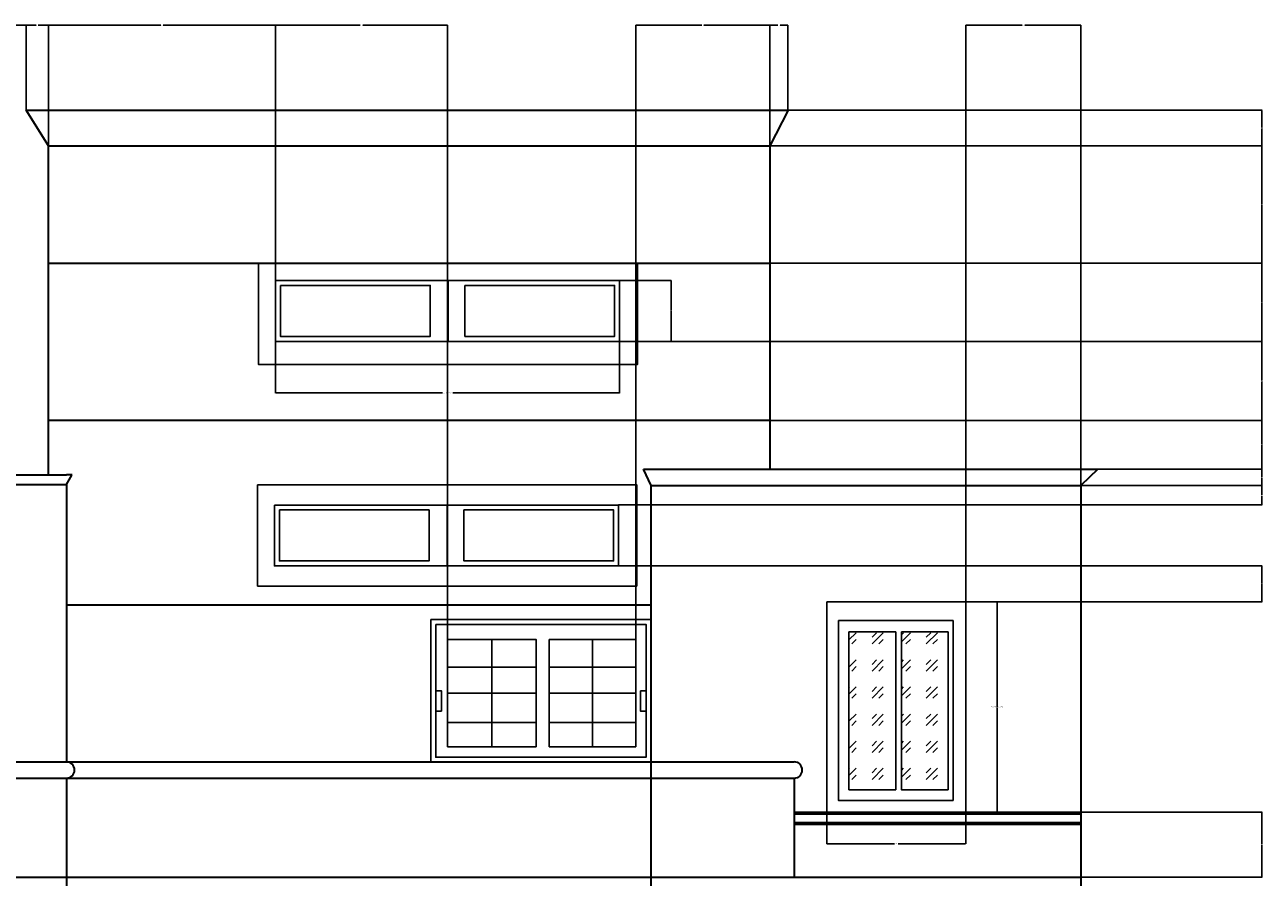
# Model space of a CAD drawing. Units: inches. Extents: x -73 to 2199, y -12 to 1583.
# Tile 3 of 3: x 686 to 2199, y 543 to 1583. Entities that reach past the tile are written whole.
import ezdxf

# ---------------------------------------------------------------- set-up
doc = ezdxf.new("R2010")
doc.units = ezdxf.units.IN
doc.header["$MEASUREMENT"] = 0
for name, color, linetype, lineweight in [('A-ANNO-DIMS', 2, 'Continuous', 18), ('A-ELEV', 7, 'Continuous', 35), ('A-GLAZ', 4, 'Continuous', 25), ('A-GLAZ-PATT', 8, 'Continuous', 13), ('A-ROOF', 7, 'Continuous', 35)]:
    doc.layers.add(name, color=color, linetype=linetype, lineweight=lineweight)
doc.styles.get("Standard").update_dxf_attribs({"font": 'arial.ttf'})
doc.dimstyles.get("Standard").update_dxf_attribs({"dimtxt": 0.75, "dimasz": 0.18, "dimexe": 0.18, "dimexo": 0.0625, "dimgap": 0.09, "dimtad": 0, "dimtih": 1, "dimtoh": 1, "dimdec": 4, "dimzin": 0, "dimdsep": 46, "dimlunit": 4, "dimtxsty": 'Standard', "dimcen": 0.09, "dimadec": 0, "dimazin": 0, "dimtfac": 1, "dimtdec": 4, "dimtofl": 0, "dimtmove": 0, "dimatfit": 3, "dimfxl": 1, "dimtolj": 1, "dimtzin": 0, "dimarcsym": 0})

# ---------------------------------------------------------------- blocks, each defined once
blk = doc.blocks.new('WIN-CASEMENT-GRID')
for p, q in [((318.2, 767.7), (318.2, 833.2)), ((441.2, 833.2), (441.2, 702.2)), ((264.1, 799.1), (372.3, 799.1)), ((388.4, 799.1), (493.9, 799.1)), ((372.3, 767.7), (264.1, 767.7)), ((318.2, 767.7), (318.2, 702.2)), ((388.4, 767.7), (493.9, 767.7)), ((264.1, 731.8), (372.3, 731.8)), ((388.4, 731.8), (493.9, 731.8))]:
    blk.add_line(p, q)
for points in [[(264.1, 833.2), (372.3, 833.2), (372.3, 702.2), (264.1, 702.2)], [(388.4, 833.2), (493.9, 833.2), (493.9, 702.2), (388.4, 702.2)]]:
    blk.add_lwpolyline(points, close=True)
blk = doc.blocks.new('WIN-STRIP')
for points in [[(992.3, 1271), (1203.2, 1271), (1203.2, 1196.7), (992.3, 1196.7)], [(1203.2, 1271), (1412.5, 1271), (1412.5, 1196.7), (1203.2, 1196.7)], [(998.3, 1265), (1181.2, 1265), (1181.2, 1202.7), (998.3, 1202.7)], [(1223.7, 1265), (1406.5, 1265), (1406.5, 1202.7), (1223.7, 1202.7)]]:
    blk.add_lwpolyline(points, close=True)
blk = doc.blocks.new('WIN-GLAZED-TALL')
for points in [[(1665.6, 878.6), (1835.3, 878.6), (1835.3, 622.1), (1665.6, 622.1)], [(1679.7, 855.9), (1819.9, 855.9), (1819.9, 636.5), (1679.7, 636.5)], [(1692.7, 842.1), (1749.8, 842.1), (1749.8, 649.4), (1692.7, 649.4)], [(1756.7, 842.1), (1813.8, 842.1), (1813.8, 649.4), (1756.7, 649.4)]]:
    blk.add_lwpolyline(points, close=True)
blk = doc.blocks.new('*D11')
at = {"layer": 'A-ANNO-DIMS', "color": 0, "lineweight": -2, "transparency": 16777216}
for p, q in [((992.3, 1196.7), (992.3, 1133.5)), ((1412.5, 1196.7), (1412.5, 1133.5)), ((992.5, 1133.7), (1196.1, 1133.7)), ((1412.3, 1133.7), (1208.8, 1133.7))]:
    blk.add_line(p, q, dxfattribs=at)
at = {"layer": 'A-ANNO-DIMS', "color": 0, "transparency": 16777216}
for points in [[(992.5, 1133.7), (992.5, 1133.7), (992.3, 1133.7)], [(1412.3, 1133.7), (1412.3, 1133.7), (1412.5, 1133.7)]]:
    blk.add_solid(points, dxfattribs=at)
at = {"layer": 'Defpoints', "color": 0, "transparency": 16777216}
for p in [(992.3, 1196.7), (1412.5, 1196.7), (1412.5, 1133.7)]:
    blk.add_point(p, dxfattribs=at)
at = {"layer": 'A-ANNO-DIMS', "color": 0, "transparency": 16777216, "insert": (1202.4, 1133.7), "char_height": 0.75, "attachment_point": 5}
blk.add_mtext('\\A1;STRIP WINDOW 420 TYP.', dxfattribs=at)
blk = doc.blocks.new('*D12')
at = {"layer": 'A-ANNO-DIMS', "color": 0, "lineweight": -2, "transparency": 16777216}
for p, q in [((1412.6, 1271), (1475.7, 1271)), ((1475.5, 1270.9), (1475.5, 1234.4)), ((1475.5, 1196.9), (1475.5, 1233.4)), ((1412.6, 1196.7), (1475.7, 1196.7))]:
    blk.add_line(p, q, dxfattribs=at)
at = {"layer": 'A-ANNO-DIMS', "color": 0, "transparency": 16777216}
for points in [[(1475.5, 1270.9), (1475.6, 1270.9), (1475.5, 1271)], [(1475.5, 1196.9), (1475.6, 1196.9), (1475.5, 1196.7)]]:
    blk.add_solid(points, dxfattribs=at)
at = {"layer": 'Defpoints', "color": 0, "transparency": 16777216}
for p in [(1412.5, 1271), (1475.5, 1271), (1412.5, 1196.7)]:
    blk.add_point(p, dxfattribs=at)
at = {"layer": 'A-ANNO-DIMS', "color": 0, "transparency": 16777216, "insert": (1475.5, 1233.9), "char_height": 0.75, "attachment_point": 5}
blk.add_mtext('\\A1;74 TYP.', dxfattribs=at)
blk = doc.blocks.new('*D13')
at = {"layer": 'A-ANNO-DIMS', "color": 0, "lineweight": -2, "transparency": 16777216}
for p, q in [((1835.4, 878.6), (1874, 878.6)), ((1873.8, 878.4), (1873.8, 750.8)), ((1873.8, 622.3), (1873.8, 749.9)), ((1835.4, 622.1), (1874, 622.1))]:
    blk.add_line(p, q, dxfattribs=at)
at = {"layer": 'A-ANNO-DIMS', "color": 0, "transparency": 16777216}
for points in [[(1873.8, 878.4), (1873.8, 878.4), (1873.8, 878.6)], [(1873.8, 622.3), (1873.8, 622.3), (1873.8, 622.1)]]:
    blk.add_solid(points, dxfattribs=at)
at = {"layer": 'Defpoints', "color": 0, "transparency": 16777216}
for p in [(1835.3, 878.6), (1873.8, 878.6), (1835.3, 622.1)]:
    blk.add_point(p, dxfattribs=at)
at = {"layer": 'A-ANNO-DIMS', "color": 0, "transparency": 16777216, "insert": (1873.8, 750.3), "char_height": 0.75, "attachment_point": 5}
blk.add_mtext('\\A1;TALL GLAZED WINDOW 257 TYP.', dxfattribs=at)
blk = doc.blocks.new('*D14')
at = {"layer": 'A-ANNO-DIMS', "color": 0, "lineweight": -2, "transparency": 16777216}
for p, q in [((1665.6, 622), (1665.6, 583.4)), ((1835.3, 622), (1835.3, 583.4)), ((1665.8, 583.6), (1748.3, 583.6)), ((1835.1, 583.6), (1752.6, 583.6))]:
    blk.add_line(p, q, dxfattribs=at)
at = {"layer": 'A-ANNO-DIMS', "color": 0, "transparency": 16777216}
for points in [[(1665.8, 583.6), (1665.8, 583.6), (1665.6, 583.6)], [(1835.1, 583.6), (1835.1, 583.6), (1835.3, 583.6)]]:
    blk.add_solid(points, dxfattribs=at)
at = {"layer": 'Defpoints', "color": 0, "transparency": 16777216}
for p in [(1665.6, 622.1), (1835.3, 622.1), (1835.3, 583.6)]:
    blk.add_point(p, dxfattribs=at)
at = {"layer": 'A-ANNO-DIMS', "color": 0, "transparency": 16777216, "insert": (1750.5, 583.6), "char_height": 0.75, "attachment_point": 5}
blk.add_mtext('\\A1;170 TYP.', dxfattribs=at)
blk = doc.blocks.new('*D27')
at = {"layer": 'A-ANNO-DIMS', "color": 0, "lineweight": -2, "transparency": 16777216}
for p, q in [((493.9, 833.2), (493.9, 1582.7)), ((494.1, 1582.6), (589.2, 1582.6)), ((687.5, 1582.6), (592.4, 1582.6)), ((687.7, 1478.9), (687.7, 1582.7))]:
    blk.add_line(p, q, dxfattribs=at)
at = {"layer": 'A-ANNO-DIMS', "color": 0, "transparency": 16777216}
for points in [[(494.1, 1582.6), (494.1, 1582.5), (493.9, 1582.6)], [(687.5, 1582.6), (687.5, 1582.5), (687.7, 1582.6)]]:
    blk.add_solid(points, dxfattribs=at)
at = {"layer": 'Defpoints', "color": 0, "transparency": 16777216}
for p in [(687.7, 1582.6), (687.7, 1478.8), (493.9, 833.2)]:
    blk.add_point(p, dxfattribs=at)
at = {"layer": 'A-ANNO-DIMS', "color": 0, "transparency": 16777216, "insert": (590.8, 1582.6), "char_height": 0.75, "attachment_point": 5}
blk.add_mtext('\\A1;193.72', dxfattribs=at)
blk = doc.blocks.new('*D28')
at = {"layer": 'A-ANNO-DIMS', "color": 0, "lineweight": -2, "transparency": 16777216}
for p, q in [((687.7, 1478.9), (687.7, 1582.7)), ((687.8, 1582.6), (699.9, 1582.6)), ((714.7, 1582.6), (702.6, 1582.6)), ((714.9, 1435.5), (714.9, 1582.7))]:
    blk.add_line(p, q, dxfattribs=at)
at = {"layer": 'A-ANNO-DIMS', "color": 0, "transparency": 16777216}
for points in [[(687.8, 1582.6), (687.8, 1582.5), (687.7, 1582.6)], [(714.7, 1582.6), (714.7, 1582.5), (714.9, 1582.6)]]:
    blk.add_solid(points, dxfattribs=at)
at = {"layer": 'Defpoints', "color": 0, "transparency": 16777216}
for p in [(714.9, 1582.6), (687.7, 1478.8), (714.9, 1435.4)]:
    blk.add_point(p, dxfattribs=at)
at = {"layer": 'A-ANNO-DIMS', "color": 0, "transparency": 16777216, "insert": (701.3, 1582.6), "char_height": 0.75, "attachment_point": 5}
blk.add_mtext('\\A1;27.27', dxfattribs=at)
blk = doc.blocks.new('*D29')
at = {"layer": 'A-ANNO-DIMS', "color": 0, "lineweight": -2, "transparency": 16777216}
for p, q in [((714.9, 1435.5), (714.9, 1582.7)), ((715.1, 1582.6), (852.3, 1582.6)), ((992.2, 1582.6), (855, 1582.6)), ((992.3, 1271.1), (992.3, 1582.7))]:
    blk.add_line(p, q, dxfattribs=at)
at = {"layer": 'A-ANNO-DIMS', "color": 0, "transparency": 16777216}
for points in [[(715.1, 1582.6), (715.1, 1582.5), (714.9, 1582.6)], [(992.2, 1582.6), (992.2, 1582.5), (992.3, 1582.6)]]:
    blk.add_solid(points, dxfattribs=at)
at = {"layer": 'Defpoints', "color": 0, "transparency": 16777216}
for p in [(992.3, 1582.6), (714.9, 1435.4), (992.3, 1271)]:
    blk.add_point(p, dxfattribs=at)
at = {"layer": 'A-ANNO-DIMS', "color": 0, "transparency": 16777216, "insert": (853.6, 1582.6), "char_height": 0.75, "attachment_point": 5}
blk.add_mtext('\\A1;277.4', dxfattribs=at)
blk = doc.blocks.new('*D30')
at = {"layer": 'A-ANNO-DIMS', "color": 0, "lineweight": -2, "transparency": 16777216}
for p, q in [((992.3, 1196.8), (992.3, 1582.7)), ((992.5, 1582.6), (1095.7, 1582.6)), ((1202.2, 1582.6), (1099, 1582.6)), ((1202.4, 833), (1202.4, 1582.7))]:
    blk.add_line(p, q, dxfattribs=at)
at = {"layer": 'A-ANNO-DIMS', "color": 0, "transparency": 16777216}
for points in [[(992.5, 1582.6), (992.5, 1582.5), (992.3, 1582.6)], [(1202.2, 1582.6), (1202.2, 1582.5), (1202.4, 1582.6)]]:
    blk.add_solid(points, dxfattribs=at)
at = {"layer": 'Defpoints', "color": 0, "transparency": 16777216}
for p in [(1202.4, 1582.6), (992.3, 1196.7), (1202.4, 833)]:
    blk.add_point(p, dxfattribs=at)
at = {"layer": 'A-ANNO-DIMS', "color": 0, "transparency": 16777216, "insert": (1097.4, 1582.6), "char_height": 0.75, "attachment_point": 5}
blk.add_mtext('\\A1;210.04', dxfattribs=at)
blk = doc.blocks.new('*D31')
at = {"layer": 'A-ANNO-DIMS', "color": 0, "lineweight": -2, "transparency": 16777216}
for p, q in [((1432.2, 833), (1432.2, 1582.7)), ((1432.4, 1582.6), (1512.9, 1582.6)), ((1596, 1582.6), (1515.5, 1582.6)), ((1596.1, 1435.5), (1596.1, 1582.7))]:
    blk.add_line(p, q, dxfattribs=at)
at = {"layer": 'A-ANNO-DIMS', "color": 0, "transparency": 16777216}
for points in [[(1432.4, 1582.6), (1432.4, 1582.5), (1432.2, 1582.6)], [(1596, 1582.6), (1596, 1582.5), (1596.1, 1582.6)]]:
    blk.add_solid(points, dxfattribs=at)
at = {"layer": 'Defpoints', "color": 0, "transparency": 16777216}
for p in [(1596.1, 1582.6), (1596.1, 1435.4), (1432.2, 833)]:
    blk.add_point(p, dxfattribs=at)
at = {"layer": 'A-ANNO-DIMS', "color": 0, "transparency": 16777216, "insert": (1514.2, 1582.6), "char_height": 0.75, "attachment_point": 5}
blk.add_mtext('\\A1;163.9', dxfattribs=at)
blk = doc.blocks.new('*D32')
at = {"layer": 'A-ANNO-DIMS', "color": 0, "lineweight": -2, "transparency": 16777216}
for p, q in [((1596.1, 1435.5), (1596.1, 1582.7)), ((1596.3, 1582.6), (1605.8, 1582.6)), ((1618.1, 1582.6), (1608.5, 1582.6)), ((1618.2, 1478.9), (1618.2, 1582.7))]:
    blk.add_line(p, q, dxfattribs=at)
at = {"layer": 'A-ANNO-DIMS', "color": 0, "transparency": 16777216}
for points in [[(1596.3, 1582.6), (1596.3, 1582.5), (1596.1, 1582.6)], [(1618.1, 1582.6), (1618.1, 1582.5), (1618.2, 1582.6)]]:
    blk.add_solid(points, dxfattribs=at)
at = {"layer": 'Defpoints', "color": 0, "transparency": 16777216}
for p in [(1618.2, 1582.6), (1618.2, 1478.8), (1596.1, 1435.4)]:
    blk.add_point(p, dxfattribs=at)
at = {"layer": 'A-ANNO-DIMS', "color": 0, "transparency": 16777216, "insert": (1607.2, 1582.6), "char_height": 0.75, "attachment_point": 5}
blk.add_mtext('\\A1;22.12', dxfattribs=at)
blk = doc.blocks.new('*D33')
at = {"layer": 'A-ANNO-DIMS', "color": 0, "lineweight": -2, "transparency": 16777216}
for p, q in [((1835.3, 878.7), (1835.3, 1582.7)), ((1835.5, 1582.6), (1904, 1582.6)), ((1975.8, 1582.6), (1907.3, 1582.6)), ((1976, 1020.6), (1976, 1582.7))]:
    blk.add_line(p, q, dxfattribs=at)
at = {"layer": 'A-ANNO-DIMS', "color": 0, "transparency": 16777216}
for points in [[(1835.5, 1582.6), (1835.5, 1582.5), (1835.3, 1582.6)], [(1975.8, 1582.6), (1975.8, 1582.5), (1976, 1582.6)]]:
    blk.add_solid(points, dxfattribs=at)
at = {"layer": 'Defpoints', "color": 0, "transparency": 16777216}
for p in [(1976, 1582.6), (1976, 1020.6), (1835.3, 878.6)]:
    blk.add_point(p, dxfattribs=at)
at = {"layer": 'A-ANNO-DIMS', "color": 0, "transparency": 16777216, "insert": (1905.6, 1582.6), "char_height": 0.75, "attachment_point": 5}
blk.add_mtext('\\A1;140.65', dxfattribs=at)
blk = doc.blocks.new('*D44')
at = {"layer": 'A-ANNO-DIMS', "color": 0, "lineweight": -2, "transparency": 16777216}
for p, q in [((1835.4, 622.1), (2197.2, 622.1)), ((2197.1, 621.9), (2197.1, 582.9)), ((2197.1, 542.9), (2197.1, 581.9)), ((1976, 542.7), (2197.2, 542.7))]:
    blk.add_line(p, q, dxfattribs=at)
at = {"layer": 'A-ANNO-DIMS', "color": 0, "transparency": 16777216}
for points in [[(2197, 621.9), (2197.1, 621.9), (2197.1, 622.1)], [(2197, 542.9), (2197.1, 542.9), (2197.1, 542.7)]]:
    blk.add_solid(points, dxfattribs=at)
at = {"layer": 'Defpoints', "color": 0, "transparency": 16777216}
for p in [(1835.3, 622.1), (2197.1, 622.1), (1976, 542.7)]:
    blk.add_point(p, dxfattribs=at)
at = {"layer": 'A-ANNO-DIMS', "color": 0, "transparency": 16777216, "insert": (2197.1, 582.4), "char_height": 0.75, "attachment_point": 5}
blk.add_mtext('\\A1;79.39', dxfattribs=at)
blk = doc.blocks.new('*D45')
at = {"layer": 'A-ANNO-DIMS', "color": 0, "lineweight": -2, "transparency": 16777216}
for p, q in [((1411.3, 922.7), (2197.2, 922.7)), ((2197.1, 922.5), (2197.1, 901.1)), ((2197.1, 878.8), (2197.1, 900.2)), ((1835.4, 878.6), (2197.2, 878.6))]:
    blk.add_line(p, q, dxfattribs=at)
at = {"layer": 'A-ANNO-DIMS', "color": 0, "transparency": 16777216}
for points in [[(2197, 922.5), (2197.1, 922.5), (2197.1, 922.7)], [(2197, 878.8), (2197.1, 878.8), (2197.1, 878.6)]]:
    blk.add_solid(points, dxfattribs=at)
at = {"layer": 'Defpoints', "color": 0, "transparency": 16777216}
for p in [(1411.2, 922.7), (2197.1, 922.7), (1835.3, 878.6)]:
    blk.add_point(p, dxfattribs=at)
at = {"layer": 'A-ANNO-DIMS', "color": 0, "transparency": 16777216, "insert": (2197.1, 900.6), "char_height": 0.75, "attachment_point": 5}
blk.add_mtext('\\A1;44.07', dxfattribs=at)
blk = doc.blocks.new('*D46')
at = {"layer": 'A-ANNO-DIMS', "color": 0, "lineweight": -2, "transparency": 16777216}
for p, q in [((1976, 1020.6), (2197.2, 1020.6)), ((2197.1, 1020.4), (2197.1, 1009.2)), ((2197.1, 997.2), (2197.1, 1008.3)), ((1411.3, 997), (2197.2, 997))]:
    blk.add_line(p, q, dxfattribs=at)
at = {"layer": 'A-ANNO-DIMS', "color": 0, "transparency": 16777216}
for points in [[(2197, 1020.4), (2197.1, 1020.4), (2197.1, 1020.6)], [(2197, 997.2), (2197.1, 997.2), (2197.1, 997)]]:
    blk.add_solid(points, dxfattribs=at)
at = {"layer": 'Defpoints', "color": 0, "transparency": 16777216}
for p in [(1976, 1020.6), (2197.1, 1020.6), (1411.2, 997)]:
    blk.add_point(p, dxfattribs=at)
at = {"layer": 'A-ANNO-DIMS', "color": 0, "transparency": 16777216, "insert": (2197.1, 1008.8), "char_height": 0.75, "attachment_point": 5}
blk.add_mtext('\\A1;23.6', dxfattribs=at)
blk = doc.blocks.new('*D47')
at = {"layer": 'A-ANNO-DIMS', "color": 0, "lineweight": -2, "transparency": 16777216}
for p, q in [((1996.6, 1040.9), (2197.2, 1040.9)), ((2197.1, 1040.7), (2197.1, 1031.2)), ((2197.1, 1020.8), (2197.1, 1030.3)), ((1976, 1020.6), (2197.2, 1020.6))]:
    blk.add_line(p, q, dxfattribs=at)
at = {"layer": 'A-ANNO-DIMS', "color": 0, "transparency": 16777216}
for points in [[(2197, 1040.7), (2197.1, 1040.7), (2197.1, 1040.9)], [(2197, 1020.8), (2197.1, 1020.8), (2197.1, 1020.6)]]:
    blk.add_solid(points, dxfattribs=at)
at = {"layer": 'Defpoints', "color": 0, "transparency": 16777216}
for p in [(1996.5, 1040.9), (2197.1, 1040.9), (1976, 1020.6)]:
    blk.add_point(p, dxfattribs=at)
at = {"layer": 'A-ANNO-DIMS', "color": 0, "transparency": 16777216, "insert": (2197.1, 1030.7), "char_height": 0.75, "attachment_point": 5}
blk.add_mtext('\\A1;20.33', dxfattribs=at)
blk = doc.blocks.new('*D48')
at = {"layer": 'A-ANNO-DIMS', "color": 0, "lineweight": -2, "transparency": 16777216}
for p, q in [((1596.2, 1100.1), (2197.2, 1100.1)), ((2197.1, 1099.9), (2197.1, 1071)), ((2197.1, 1041.1), (2197.1, 1070)), ((1996.6, 1040.9), (2197.2, 1040.9))]:
    blk.add_line(p, q, dxfattribs=at)
at = {"layer": 'A-ANNO-DIMS', "color": 0, "transparency": 16777216}
for points in [[(2197, 1099.9), (2197.1, 1099.9), (2197.1, 1100.1)], [(2197, 1041.1), (2197.1, 1041.1), (2197.1, 1040.9)]]:
    blk.add_solid(points, dxfattribs=at)
at = {"layer": 'Defpoints', "color": 0, "transparency": 16777216}
for p in [(1596.1, 1100.1), (2197.1, 1100.1), (1996.5, 1040.9)]:
    blk.add_point(p, dxfattribs=at)
at = {"layer": 'A-ANNO-DIMS', "color": 0, "transparency": 16777216, "insert": (2197.1, 1070.5), "char_height": 0.75, "attachment_point": 5}
blk.add_mtext('\\A1;59.18', dxfattribs=at)
blk = doc.blocks.new('*D49')
at = {"layer": 'A-ANNO-DIMS', "color": 0, "lineweight": -2, "transparency": 16777216}
for p, q in [((1412.6, 1196.7), (2197.2, 1196.7)), ((2197.1, 1196.6), (2197.1, 1148.9)), ((2197.1, 1100.3), (2197.1, 1147.9)), ((1596.2, 1100.1), (2197.2, 1100.1))]:
    blk.add_line(p, q, dxfattribs=at)
at = {"layer": 'A-ANNO-DIMS', "color": 0, "transparency": 16777216}
for points in [[(2197, 1196.6), (2197.1, 1196.6), (2197.1, 1196.7)], [(2197, 1100.3), (2197.1, 1100.3), (2197.1, 1100.1)]]:
    blk.add_solid(points, dxfattribs=at)
at = {"layer": 'Defpoints', "color": 0, "transparency": 16777216}
for p in [(1412.5, 1196.7), (2197.1, 1196.7), (1596.1, 1100.1)]:
    blk.add_point(p, dxfattribs=at)
at = {"layer": 'A-ANNO-DIMS', "color": 0, "transparency": 16777216, "insert": (2197.1, 1148.4), "char_height": 0.75, "attachment_point": 5}
blk.add_mtext('\\A1;96.65', dxfattribs=at)
blk = doc.blocks.new('*D50')
at = {"layer": 'A-ANNO-DIMS', "color": 0, "lineweight": -2, "transparency": 16777216}
for p, q in [((1596.2, 1292.3), (2197.2, 1292.3)), ((2197.1, 1292.1), (2197.1, 1245)), ((2197.1, 1196.9), (2197.1, 1244)), ((1412.6, 1196.7), (2197.2, 1196.7))]:
    blk.add_line(p, q, dxfattribs=at)
at = {"layer": 'A-ANNO-DIMS', "color": 0, "transparency": 16777216}
for points in [[(2197, 1292.1), (2197.1, 1292.1), (2197.1, 1292.3)], [(2197, 1196.9), (2197.1, 1196.9), (2197.1, 1196.7)]]:
    blk.add_solid(points, dxfattribs=at)
at = {"layer": 'Defpoints', "color": 0, "transparency": 16777216}
for p in [(1596.1, 1292.3), (2197.1, 1292.3), (1412.5, 1196.7)]:
    blk.add_point(p, dxfattribs=at)
at = {"layer": 'A-ANNO-DIMS', "color": 0, "transparency": 16777216, "insert": (2197.1, 1244.5), "char_height": 0.75, "attachment_point": 5}
blk.add_mtext('\\A1;95.53', dxfattribs=at)
blk = doc.blocks.new('*D51')
at = {"layer": 'A-ANNO-DIMS', "color": 0, "lineweight": -2, "transparency": 16777216}
for p, q in [((1596.2, 1435.4), (2197.2, 1435.4)), ((2197.1, 1435.2), (2197.1, 1364.3)), ((2197.1, 1292.4), (2197.1, 1363.4)), ((1596.2, 1292.3), (2197.2, 1292.3))]:
    blk.add_line(p, q, dxfattribs=at)
at = {"layer": 'A-ANNO-DIMS', "color": 0, "transparency": 16777216}
for points in [[(2197, 1435.2), (2197.1, 1435.2), (2197.1, 1435.4)], [(2197, 1292.4), (2197.1, 1292.4), (2197.1, 1292.3)]]:
    blk.add_solid(points, dxfattribs=at)
at = {"layer": 'Defpoints', "color": 0, "transparency": 16777216}
for p in [(1596.1, 1435.4), (2197.1, 1435.4), (1596.1, 1292.3)]:
    blk.add_point(p, dxfattribs=at)
at = {"layer": 'A-ANNO-DIMS', "color": 0, "transparency": 16777216, "insert": (2197.1, 1363.8), "char_height": 0.75, "attachment_point": 5}
blk.add_mtext('\\A1;143.14', dxfattribs=at)
blk = doc.blocks.new('*D52')
at = {"layer": 'A-ANNO-DIMS', "color": 0, "lineweight": -2, "transparency": 16777216}
for p, q in [((1618.3, 1478.8), (2197.2, 1478.8)), ((2197.1, 1478.6), (2197.1, 1457.6)), ((2197.1, 1435.6), (2197.1, 1456.6)), ((1596.2, 1435.4), (2197.2, 1435.4))]:
    blk.add_line(p, q, dxfattribs=at)
at = {"layer": 'A-ANNO-DIMS', "color": 0, "transparency": 16777216}
for points in [[(2197, 1478.6), (2197.1, 1478.6), (2197.1, 1478.8)], [(2197, 1435.6), (2197.1, 1435.6), (2197.1, 1435.4)]]:
    blk.add_solid(points, dxfattribs=at)
at = {"layer": 'Defpoints', "color": 0, "transparency": 16777216}
for p in [(1618.2, 1478.8), (2197.1, 1478.8), (1596.1, 1435.4)]:
    blk.add_point(p, dxfattribs=at)
at = {"layer": 'A-ANNO-DIMS', "color": 0, "transparency": 16777216, "insert": (2197.1, 1457.1), "char_height": 0.75, "attachment_point": 5}
blk.add_mtext('\\A1;43.41', dxfattribs=at)

msp = doc.modelspace()

# ---------------------------------------------------------------- hatches: boundary and pattern name
at = {"layer": 'A-GLAZ-PATT'}
h = msp.add_hatch(dxfattribs=at)
h.set_pattern_fill('GOST_GLASS', color=256, scale=3.9)
h.set_pattern_definition([(45, (0, 0), (33.0926, 0), [19.5, -27.3]), (45, (8.273, 0), (33.0926, 0), [7.8, -39]), (45, (0, 8.273), (33.0926, 0), [7.8, -39])])
h.paths.add_polyline_path([(1813.8199, 842.1341), (1756.6853, 842.1341), (1756.6853, 649.4087), (1813.8199, 649.4087)])
h.paths.add_polyline_path([(1749.7931, 842.1341), (1692.6585, 842.1341), (1692.6585, 649.4087), (1749.7931, 649.4087)])
h.paths.add_polyline_path([(1813.8199, 414.5003), (1756.6853, 414.5003), (1756.6853, 221.7748), (1813.8199, 221.7748)])
h.paths.add_polyline_path([(1749.7931, 414.5003), (1692.6585, 414.5003), (1692.6585, 221.7748), (1749.7931, 221.7748)])

# ---------------------------------------------------------------- linework, layer by layer
at = {"layer": 'A-ELEV'}
for p, q in [((714.9232, 1033.8877), (714.9232, 1435.4098)), ((714.9232, 1435.4098), (1596.1301, 1435.4098)), ((1596.1301, 1435.4098), (1596.1301, 1040.9027)), ((714.9232, 1292.2662), (714.9232, 1292.2662)), ((714.9232, 1292.2662), (1596.1301, 1292.2662)), ((1596.1301, 1100.0837), (714.9232, 1100.0837)), ((42.6128, 1033.8877), (736.9068, 1033.8877)), ((42.6128, 1021.8877), (736.9068, 1021.8877)), ((736.9068, 1021.8877), (736.9068, 683.3913)), ((736.9068, 875.1658), (1450.9568, 875.1658)), ((42.6128, 683.3913), (736.9068, 683.3913)), ((736.9068, 683.3913), (1625.7698, 683.3913)), ((42.6128, 663.5939), (736.9068, 663.5939)), ((736.9068, 663.5939), (736.9068, 542.7065)), ((736.9068, 663.5939), (1625.7698, 663.5939)), ((1625.7698, 663.5939), (1625.7698, 542.7065)), ((1625.7698, 622.0942), (1975.9662, 622.0942)), ((1625.7698, 620.0942), (1975.9662, 620.0942)), ((1625.7698, 609.3386), (1975.9662, 609.3386)), ((1625.7698, 607.3386), (1975.9662, 607.3386)), ((42.6128, 542.7065), (736.9068, 542.7065)), ((736.9068, 542.7065), (736.9068, 131.0114)), ((736.9068, 542.7065), (1625.7698, 542.7065)), ((1625.7698, 542.7065), (1975.9662, 542.7065))]:
    msp.add_line(p, q, dxfattribs=at)
msp.add_lwpolyline([(1450.9568, 1020.5741), (1975.9662, 1020.5741), (1975.9662, 131.0114), (1450.9568, 131.0114)], close=True, dxfattribs=at)
for centre in [(736.9068, 673.4926), (1625.7698, 673.4926)]:
    msp.add_arc(centre, 9.8987, 270, 90, dxfattribs=at)
at = {"layer": 'A-GLAZ'}
for points in [[(971.325, 1292.2662), (1434.4229, 1292.2662), (1434.4229, 1168.6226), (971.325, 1168.6226)], [(970.3876, 1021.6448), (1433.4854, 1021.6448), (1433.4854, 898.0011), (970.3876, 898.0011)], [(1181.9595, 857.2194), (1450.9568, 857.2194), (1450.9568, 683.1886), (1181.9595, 683.1886)], [(1187.9595, 851.2194), (1444.9568, 851.2194), (1444.9568, 689.1886), (1187.9595, 689.1886)], [(1187.9595, 770.204), (1194.8707, 770.204), (1194.8707, 745.3915), (1187.9595, 745.3915)], [(1438.0456, 770.204), (1444.9568, 770.204), (1444.9568, 745.3915), (1438.0456, 745.3915)]]:
    msp.add_lwpolyline(points, close=True, dxfattribs=at)
at = {"layer": 'A-ROOF'}
for p, q in [((714.9232, 1435.4098), (687.6523, 1478.8169)), ((687.6523, 1478.8169), (1618.2482, 1478.8169)), ((1618.2482, 1478.8169), (1596.1301, 1435.4098)), ((743.81, 1033.8877), (736.9068, 1033.8877)), ((736.9068, 1021.8877), (743.4963, 1033.4238)), ((743.4963, 1033.4238), (743.81, 1033.8877)), ((1450.9568, 1020.5741), (1441.5877, 1040.9027)), ((1441.5877, 1040.9027), (1996.5385, 1040.9027)), ((1996.5385, 1040.9027), (1975.9662, 1020.5741))]:
    msp.add_line(p, q, dxfattribs=at)

# ---------------------------------------------------------------- block references
at = {"layer": 'A-GLAZ'}
for name, p in [('WIN-STRIP', (0, 0)), ('WIN-STRIP', (-1.2929, -274.0626)), ('WIN-GLAZED-TALL', (0, 0)), ('WIN-CASEMENT-GRID', (938.3152, -0.2026))]:
    msp.add_blockref(name, p, dxfattribs=at)

# ---------------------------------------------------------------- dimensions: what is measured, and where the dimension line sits
at = {"layer": 'A-ANNO-DIMS'}
for base, p1, p2, override, picture, middle in [((687.6523, 1582.5669), (493.9311, 833.1626), (687.6523, 1478.8169), {"dimdec": 2, "dimlfac": 1, "dimrnd": 0, "dimzin": 0, "dimdsep": 46, "dimlunit": 2}, '*D27', (590.7917, 1582.5669)), ((714.9232, 1582.5669), (687.6523, 1478.8169), (714.9232, 1435.4098), {"dimdec": 2, "dimlfac": 1, "dimrnd": 0, "dimzin": 0, "dimdsep": 46, "dimlunit": 2}, '*D28', (701.2877, 1582.5669)), ((992.3411, 1582.5669), (714.9232, 1435.4098), (992.3411, 1271.0378), {"dimdec": 1, "dimlfac": 1, "dimrnd": 0, "dimzin": 0, "dimdsep": 46, "dimlunit": 2}, '*D29', (853.6321, 1582.5669)), ((1202.3822, 1582.5669), (992.3411, 1196.7332), (1202.3822, 832.96), {"dimdec": 2, "dimlfac": 1, "dimrnd": 0, "dimzin": 0, "dimdsep": 46, "dimlunit": 2}, '*D30', (1097.3616, 1582.5669)), ((1596.1301, 1582.5669), (1432.2462, 832.96), (1596.1301, 1435.4098), {"dimdec": 1, "dimlfac": 1, "dimrnd": 0, "dimzin": 0, "dimdsep": 46, "dimlunit": 2}, '*D31', (1514.1882, 1582.5669)), ((1618.2482, 1582.5669), (1596.1301, 1435.4098), (1618.2482, 1478.8169), {"dimdec": 2, "dimlfac": 1, "dimrnd": 0, "dimzin": 0, "dimdsep": 46, "dimlunit": 2}, '*D32', (1607.1891, 1582.5669)), ((1975.9662, 1582.5669), (1835.312, 878.5968), (1975.9662, 1020.5741), {"dimdec": 2, "dimlfac": 1, "dimrnd": 0, "dimzin": 0, "dimdsep": 46, "dimlunit": 2}, '*D33', (1905.6391, 1582.5669))]:
    dim = msp.add_linear_dim(base=base, p1=p1, p2=p2, dimstyle='Standard', override=override, dxfattribs=at)
    dim.commit()
    dim.dimension.update_dxf_attribs({"geometry": picture, "text_midpoint": middle})
for base, p1, p2, override, picture, middle in [((2197.0526, 1478.8169), (1596.1301, 1435.4098), (1618.2482, 1478.8169), {"dimdec": 2, "dimlfac": 1, "dimrnd": 0, "dimzin": 0, "dimdsep": 46, "dimlunit": 2}, '*D52', (2197.0526, 1457.1134)), ((2197.0526, 1435.4098), (1596.1301, 1292.2662), (1596.1301, 1435.4098), {"dimdec": 2, "dimlfac": 1, "dimrnd": 0, "dimzin": 0, "dimdsep": 46, "dimlunit": 2}, '*D51', (2197.0526, 1363.838)), ((2197.0526, 1292.2662), (1412.499, 1196.7332), (1596.1301, 1292.2662), {"dimdec": 2, "dimlfac": 1, "dimrnd": 0, "dimzin": 0, "dimdsep": 46, "dimlunit": 2}, '*D50', (2197.0526, 1244.4997)), ((2197.0526, 1196.7332), (1596.1301, 1100.0837), (1412.499, 1196.7332), {"dimdec": 2, "dimlfac": 1, "dimrnd": 0, "dimzin": 0, "dimdsep": 46, "dimlunit": 2}, '*D49', (2197.0526, 1148.4084)), ((2197.0526, 1100.0837), (1996.5385, 1040.9027), (1596.1301, 1100.0837), {"dimdec": 2, "dimlfac": 1, "dimrnd": 0, "dimzin": 0, "dimdsep": 46, "dimlunit": 2}, '*D48', (2197.0526, 1070.4932)), ((2197.0526, 1040.9027), (1975.9662, 1020.5741), (1996.5385, 1040.9027), {"dimdec": 2, "dimlfac": 1, "dimrnd": 0, "dimzin": 0, "dimdsep": 46, "dimlunit": 2}, '*D47', (2197.0526, 1030.7384)), ((2197.0526, 1020.5741), (1411.2061, 996.9753), (1975.9662, 1020.5741), {"dimdec": 1, "dimlfac": 1, "dimrnd": 0, "dimzin": 0, "dimdsep": 46, "dimlunit": 2}, '*D46', (2197.0526, 1008.7747)), ((2197.0526, 922.6706), (1835.312, 878.5968), (1411.2061, 922.6706), {"dimdec": 2, "dimlfac": 1, "dimrnd": 0, "dimzin": 0, "dimdsep": 46, "dimlunit": 2}, '*D45', (2197.0526, 900.6337)), ((2197.0526, 622.0942), (1975.9662, 542.7065), (1835.312, 622.0942), {"dimdec": 2, "dimlfac": 1, "dimrnd": 0, "dimzin": 0, "dimdsep": 46, "dimlunit": 2}, '*D44', (2197.0526, 582.4004))]:
    dim = msp.add_linear_dim(base=base, p1=p1, p2=p2, angle=90, dimstyle='Standard', override=override, dxfattribs=at)
    dim.commit()
    dim.dimension.update_dxf_attribs({"geometry": picture, "text_midpoint": middle})
for base, p1, p2, text, picture, middle in [((1475.5227, 1271.0378), (1412.499, 1196.7332), (1412.499, 1271.0378), '<> TYP.', '*D12', (1475.5227, 1233.8855)), ((1873.7874, 878.5968), (1835.312, 622.0942), (1835.312, 878.5968), 'TALL GLAZED WINDOW <> TYP.', '*D13', (1873.7874, 750.3455))]:
    dim = msp.add_linear_dim(base=base, p1=p1, p2=p2, angle=90, text=text, dimstyle='Standard', override={"dimdec": 0, "dimlfac": 1, "dimrnd": 0, "dimzin": 0, "dimdsep": 46, "dimlunit": 2}, dxfattribs=at)
    dim.commit()
    dim.dimension.update_dxf_attribs({"geometry": picture, "text_midpoint": middle})
for base, p1, p2, text, picture, middle in [((1412.499, 1133.7095), (992.3411, 1196.7332), (1412.499, 1196.7332), 'STRIP WINDOW <> TYP.', '*D11', (1202.4201, 1133.7095)), ((1835.312, 583.6188), (1665.5962, 622.0942), (1835.312, 622.0942), '<> TYP.', '*D14', (1750.4541, 583.6188))]:
    dim = msp.add_linear_dim(base=base, p1=p1, p2=p2, text=text, dimstyle='Standard', override={"dimdec": 0, "dimlfac": 1, "dimrnd": 0, "dimzin": 0, "dimdsep": 46, "dimlunit": 2}, dxfattribs=at)
    dim.commit()
    dim.dimension.update_dxf_attribs({"geometry": picture, "text_midpoint": middle})

doc.saveas('drawing.dxf')
